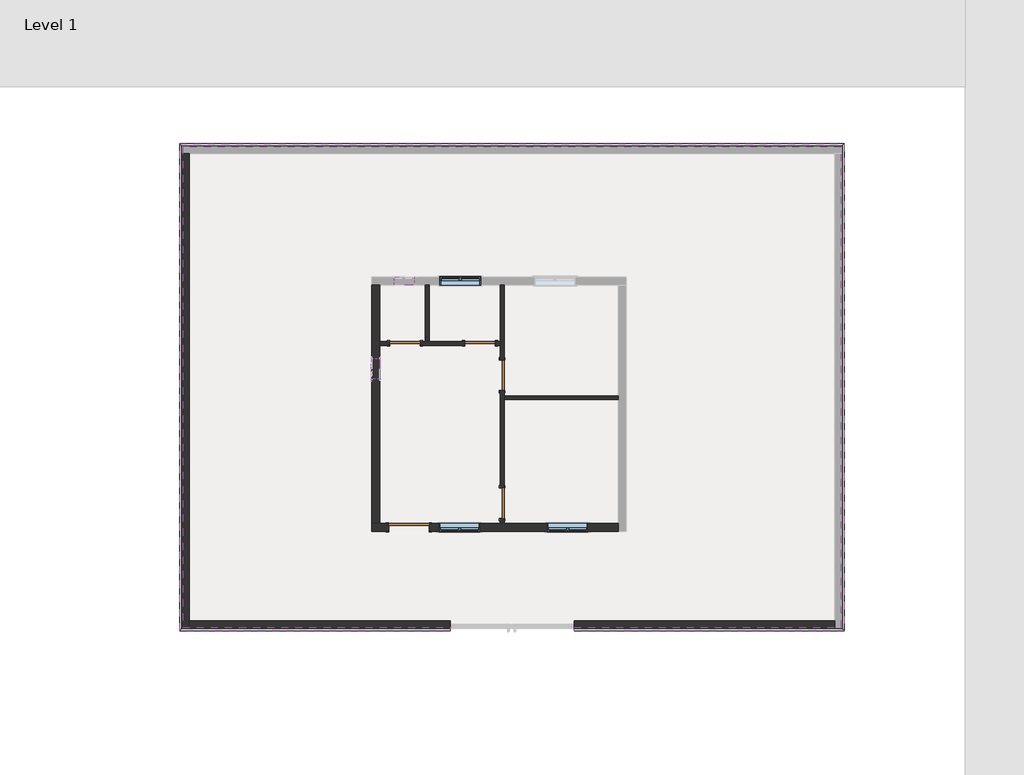
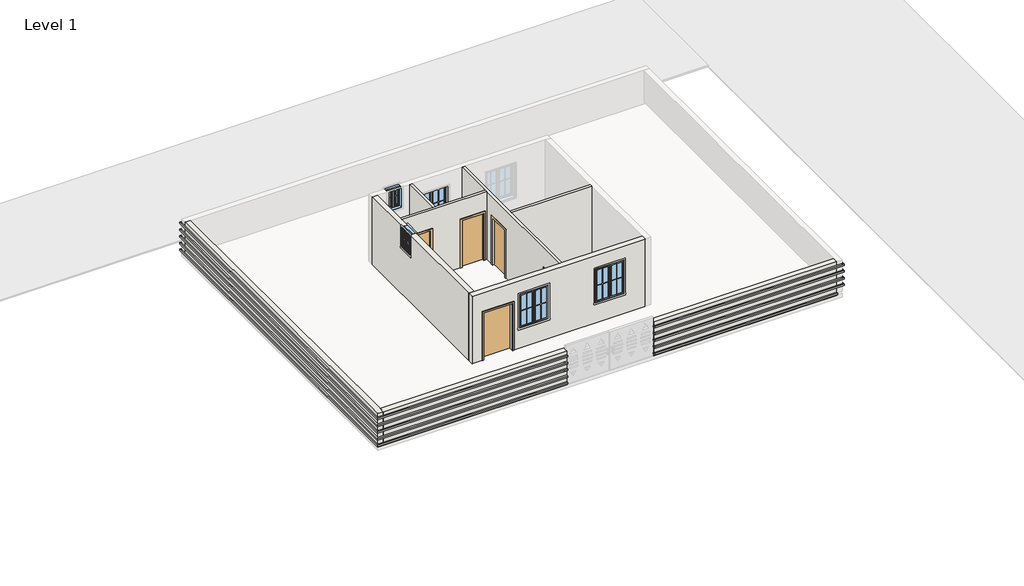
# One storey, part 1 of 2: 9 walls, 5 doors, 5 proxies, 5 windows.
"""IFC4 building model written with IfcOpenShell, lengths in millimetres."""

from ifc_helpers import new_model, si_unit, frame, origin, origin_with_axes, place, context, project, spatial, polyline, outline, extrude, faceted_brep, transform, mapped, element, save
from components import door_e5f9f3c4, door_f4c4cdf2, window_c417fced, window_8377141f

model = new_model("IFC4")

# Units and contexts
model_context = context("Model", 3, world=origin())
ifc_project = project(units=[si_unit("LENGTHUNIT", "METRE", prefix="MILLI")], contexts=[model_context])

# Site, building, storey
site = spatial("IfcSite", under=ifc_project)
building = spatial("IfcBuilding", under=site)
storey = spatial("IfcBuildingStorey", under=building, Name="Level 1", Elevation=0.0)

# Proxies
placement = place(None, origin())
element("IfcBuildingElementProxy", 1, Name="Reveal", ObjectType="Reveal", at=placement, inside=storey, context=model_context, shape_type="SweptSolid", body=[
    extrude(outline(polyline([(3367.5654616, 3455.855505), (3367.5654616, 3363.780505), (-4756.9239856, 3363.780505), (-4664.8489856, 3455.855505), (3367.5654616, 3455.855505)])), frame((0.0, 0.0, 76.2), z_axis=(0.0, 0.0, 1.0), x_axis=(1.0, 0.0, 0.0)), (0.0, 0.0, 1.0), 67.7333333),
    extrude(outline(polyline([(14893.1510144, 3455.855505), (14893.1510144, 3363.780505), (7082.6510144, 3363.780505), (7082.6510144, 3455.855505), (14893.1510144, 3455.855505)])), frame((0.0, 0.0, 76.2), z_axis=(0.0, 0.0, 1.0), x_axis=(1.0, 0.0, 0.0)), (0.0, 0.0, 1.0), 67.7333333),
    extrude(outline(polyline([(-4664.8489856, 17883.055505), (-4756.9239856, 17975.130505), (15121.7510144, 17975.130505), (15121.7510144, 17883.055505), (-4664.8489856, 17883.055505)])), frame((0.0, 0.0, 76.2), z_axis=(0.0, 0.0, 1.0), x_axis=(1.0, 0.0, 0.0)), (0.0, 0.0, 1.0), 67.7333333),
    extrude(outline(polyline([(-4664.8489856, 3455.855505), (-4756.9239856, 3363.780505), (-4756.9239856, 17975.130505), (-4664.8489856, 17883.055505), (-4664.8489856, 3455.855505)])), frame((0.0, 0.0, 76.2), z_axis=(0.0, 0.0, 1.0), x_axis=(1.0, 0.0, 0.0)), (0.0, 0.0, 1.0), 67.7333333),
])
element("IfcBuildingElementProxy", 2, Name="Reveal", ObjectType="Reveal", at=placement, inside=storey, context=model_context, shape_type="SweptSolid", body=[
    extrude(outline(polyline([(3367.5654616, 3455.855505), (3367.5654616, 3363.780505), (-4756.9239856, 3363.780505), (-4664.8489856, 3455.855505), (3367.5654616, 3455.855505)])), frame((0.0, 0.0, 381.0), z_axis=(0.0, 0.0, 1.0), x_axis=(1.0, 0.0, 0.0)), (0.0, 0.0, 1.0), 67.7333333),
    extrude(outline(polyline([(15096.3510144, 3455.855505), (15188.4260144, 3363.780505), (7082.6510144, 3363.780505), (7082.6510144, 3455.855505), (15096.3510144, 3455.855505)])), frame((0.0, 0.0, 381.0), z_axis=(0.0, 0.0, 1.0), x_axis=(1.0, 0.0, 0.0)), (0.0, 0.0, 1.0), 67.7333333),
    extrude(outline(polyline([(15096.3510144, 17883.055505), (15188.4260144, 17975.130505), (15188.4260144, 3363.780505), (15096.3510144, 3455.855505), (15096.3510144, 17883.055505)])), frame((0.0, 0.0, 381.0), z_axis=(0.0, 0.0, 1.0), x_axis=(1.0, 0.0, 0.0)), (0.0, 0.0, 1.0), 67.7333333),
    extrude(outline(polyline([(-4664.8489856, 17883.055505), (-4756.9239856, 17975.130505), (15188.4260144, 17975.130505), (15096.3510144, 17883.055505), (-4664.8489856, 17883.055505)])), frame((0.0, 0.0, 381.0), z_axis=(0.0, 0.0, 1.0), x_axis=(1.0, 0.0, 0.0)), (0.0, 0.0, 1.0), 67.7333333),
    extrude(outline(polyline([(-4664.8489856, 3455.855505), (-4756.9239856, 3363.780505), (-4756.9239856, 17975.130505), (-4664.8489856, 17883.055505), (-4664.8489856, 3455.855505)])), frame((0.0, 0.0, 381.0), z_axis=(0.0, 0.0, 1.0), x_axis=(1.0, 0.0, 0.0)), (0.0, 0.0, 1.0), 67.7333333),
])
element("IfcBuildingElementProxy", 3, Name="Reveal", ObjectType="Reveal", at=placement, inside=storey, context=model_context, shape_type="SweptSolid", body=[
    extrude(outline(polyline([(3367.5654616, 3455.855505), (3367.5654616, 3363.780505), (-4756.9239856, 3363.780505), (-4664.8489856, 3455.855505), (3367.5654616, 3455.855505)])), frame((0.0, 0.0, 685.8), z_axis=(0.0, 0.0, 1.0), x_axis=(1.0, 0.0, 0.0)), (0.0, 0.0, 1.0), 67.7333333),
    extrude(outline(polyline([(15096.3510144, 3455.855505), (15188.4260144, 3363.780505), (7082.6510144, 3363.780505), (7082.6510144, 3455.855505), (15096.3510144, 3455.855505)])), frame((0.0, 0.0, 685.8), z_axis=(0.0, 0.0, 1.0), x_axis=(1.0, 0.0, 0.0)), (0.0, 0.0, 1.0), 67.7333333),
    extrude(outline(polyline([(15096.3510144, 17883.055505), (15188.4260144, 17975.130505), (15188.4260144, 3363.780505), (15096.3510144, 3455.855505), (15096.3510144, 17883.055505)])), frame((0.0, 0.0, 685.8), z_axis=(0.0, 0.0, 1.0), x_axis=(1.0, 0.0, 0.0)), (0.0, 0.0, 1.0), 67.7333333),
    extrude(outline(polyline([(-4664.8489856, 17883.055505), (-4756.9239856, 17975.130505), (15188.4260144, 17975.130505), (15096.3510144, 17883.055505), (-4664.8489856, 17883.055505)])), frame((0.0, 0.0, 685.8), z_axis=(0.0, 0.0, 1.0), x_axis=(1.0, 0.0, 0.0)), (0.0, 0.0, 1.0), 67.7333333),
    extrude(outline(polyline([(-4664.8489856, 3455.855505), (-4756.9239856, 3363.780505), (-4756.9239856, 17975.130505), (-4664.8489856, 17883.055505), (-4664.8489856, 3455.855505)])), frame((0.0, 0.0, 685.8), z_axis=(0.0, 0.0, 1.0), x_axis=(1.0, 0.0, 0.0)), (0.0, 0.0, 1.0), 67.7333333),
])
element("IfcBuildingElementProxy", 4, Name="Reveal", ObjectType="Reveal", at=placement, inside=storey, context=model_context, shape_type="SweptSolid", body=[
    extrude(outline(polyline([(3367.5654616, 3455.855505), (3367.5654616, 3363.780505), (-4756.9239856, 3363.780505), (-4664.8489856, 3455.855505), (3367.5654616, 3455.855505)])), frame((0.0, 0.0, 990.6), z_axis=(0.0, 0.0, 1.0), x_axis=(1.0, 0.0, 0.0)), (0.0, 0.0, 1.0), 67.7333333),
    extrude(outline(polyline([(15096.3510144, 3455.855505), (15188.4260144, 3363.780505), (7082.6510144, 3363.780505), (7082.6510144, 3455.855505), (15096.3510144, 3455.855505)])), frame((0.0, 0.0, 990.6), z_axis=(0.0, 0.0, 1.0), x_axis=(1.0, 0.0, 0.0)), (0.0, 0.0, 1.0), 67.7333333),
    extrude(outline(polyline([(15096.3510144, 17883.055505), (15188.4260144, 17975.130505), (15188.4260144, 3363.780505), (15096.3510144, 3455.855505), (15096.3510144, 17883.055505)])), frame((0.0, 0.0, 990.6), z_axis=(0.0, 0.0, 1.0), x_axis=(1.0, 0.0, 0.0)), (0.0, 0.0, 1.0), 67.7333333),
    extrude(outline(polyline([(-4664.8489856, 17883.055505), (-4756.9239856, 17975.130505), (15188.4260144, 17975.130505), (15096.3510144, 17883.055505), (-4664.8489856, 17883.055505)])), frame((0.0, 0.0, 990.6), z_axis=(0.0, 0.0, 1.0), x_axis=(1.0, 0.0, 0.0)), (0.0, 0.0, 1.0), 67.7333333),
    extrude(outline(polyline([(-4664.8489856, 3455.855505), (-4756.9239856, 3363.780505), (-4756.9239856, 17975.130505), (-4664.8489856, 17883.055505), (-4664.8489856, 3455.855505)])), frame((0.0, 0.0, 990.6), z_axis=(0.0, 0.0, 1.0), x_axis=(1.0, 0.0, 0.0)), (0.0, 0.0, 1.0), 67.7333333),
])
element("IfcBuildingElementProxy", 5, Name="Reveal", ObjectType="Reveal", at=placement, inside=storey, context=model_context, shape_type="SweptSolid", body=[
    extrude(outline(polyline([(3367.5654616, 3455.855505), (3367.5654616, 3363.780505), (-4756.9239856, 3363.780505), (-4664.8489856, 3455.855505), (3367.5654616, 3455.855505)])), frame((0.0, 0.0, 1295.4), z_axis=(0.0, 0.0, 1.0), x_axis=(1.0, 0.0, 0.0)), (0.0, 0.0, 1.0), 67.7333333),
    extrude(outline(polyline([(15096.3510144, 3455.855505), (15188.4260144, 3363.780505), (7082.6510144, 3363.780505), (7082.6510144, 3455.855505), (15096.3510144, 3455.855505)])), frame((0.0, 0.0, 1295.4), z_axis=(0.0, 0.0, 1.0), x_axis=(1.0, 0.0, 0.0)), (0.0, 0.0, 1.0), 67.7333333),
    extrude(outline(polyline([(15096.3510144, 17883.055505), (15188.4260144, 17975.130505), (15188.4260144, 3363.780505), (15096.3510144, 3455.855505), (15096.3510144, 17883.055505)])), frame((0.0, 0.0, 1295.4), z_axis=(0.0, 0.0, 1.0), x_axis=(1.0, 0.0, 0.0)), (0.0, 0.0, 1.0), 67.7333333),
    extrude(outline(polyline([(-4664.8489856, 17883.055505), (-4756.9239856, 17975.130505), (15188.4260144, 17975.130505), (15096.3510144, 17883.055505), (-4664.8489856, 17883.055505)])), frame((0.0, 0.0, 1295.4), z_axis=(0.0, 0.0, 1.0), x_axis=(1.0, 0.0, 0.0)), (0.0, 0.0, 1.0), 67.7333333),
    extrude(outline(polyline([(-4664.8489856, 3455.855505), (-4756.9239856, 3363.780505), (-4756.9239856, 17975.130505), (-4664.8489856, 17883.055505), (-4664.8489856, 3455.855505)])), frame((0.0, 0.0, 1295.4), z_axis=(0.0, 0.0, 1.0), x_axis=(1.0, 0.0, 0.0)), (0.0, 0.0, 1.0), 67.7333333),
])

# Doors
door_shape = door_e5f9f3c4(model_context)
element("IfcDoor", 6, ObjectType="Single-Flush : 36\" x 84\"", at=placement, inside=storey, context=model_context, shape_type="MappedRepresentation", body=[
    mapped(door_shape, transform((2006.6, 11982.45, 0.0), x_axis=(1.0, 0.0, 0.0), y_axis=(0.0, 1.0, 0.0), z_axis=(0.0, 0.0, 1.0))),
])
element("IfcDoor", 7, ObjectType="Single-Flush : 36\" x 84\"", at=placement, inside=storey, context=model_context, shape_type="MappedRepresentation", body=[
    mapped(door_shape, transform((4254.5, 11982.45, 0.0), x_axis=(1.0, 0.0, 0.0), y_axis=(0.0, 1.0, 0.0), z_axis=(0.0, 0.0, 1.0))),
])
element("IfcDoor", 8, ObjectType="Single-Flush : 36\" x 84\"", at=placement, inside=storey, context=model_context, shape_type="MappedRepresentation", body=[
    mapped(door_shape, transform((4921.25, 11023.6, 0.0), x_axis=(0.0, -1.0, 0.0), y_axis=(1.0, 0.0, 0.0), z_axis=(0.0, 0.0, 1.0))),
])
element("IfcDoor", 9, ObjectType="Single-Flush : 36\" x 84\"", at=placement, inside=storey, context=model_context, shape_type="MappedRepresentation", body=[
    mapped(door_shape, transform((4921.25, 7188.2, 0.0), x_axis=(0.0, -1.0, 0.0), y_axis=(1.0, 0.0, 0.0), z_axis=(0.0, 0.0, 1.0))),
])
door_2_shape = door_f4c4cdf2(model_context)
element("IfcDoor", 10, ObjectType="Single-Flush : 48\" x 84\"", at=placement, inside=storey, context=model_context, shape_type="MappedRepresentation", body=[
    mapped(door_2_shape, transform((2120.9, 6464.3, 0.0), x_axis=(-1.0, 0.0, 0.0), y_axis=(0.0, -1.0, 0.0), z_axis=(0.0, 0.0, 1.0))),
])

# Walls
element("IfcWall", 11, ObjectType="Generic - 5\"", at=placement, inside=storey, context=model_context, shape_type="SweptSolid", body=[
    extrude(outline(polyline([(2616.2, 12039.6), (2616.2, 13741.4), (2730.5, 13741.4), (2730.5, 12039.6), (2616.2, 12039.6)])), origin_with_axes(), (0.0, 0.0, 1.0), 3048.0),
])
element("IfcWall", 12, ObjectType="Generic - 5\"", at=placement, inside=storey, context=model_context, shape_type="Brep", body=[
    faceted_brep([(4711.7, 11925.3, 2133.6), (4711.7, 11925.3, 0.0), (4864.1, 11925.3, 0.0), (4864.1, 11925.3, 3048.0), (1244.6, 11925.3, 3048.0), (1244.6, 11925.3, 0.0), (1549.4, 11925.3, 0.0), (1549.4, 11925.3, 2133.6), (2463.8, 11925.3, 2133.6), (2463.8, 11925.3, 0.0), (3797.3, 11925.3, 0.0), (3797.3, 11925.3, 2133.6), (4864.1, 12039.6, 0.0), (4711.7, 12039.6, 0.0), (4711.7, 12039.6, 2133.6), (3797.3, 12039.6, 2133.6), (3797.3, 12039.6, 0.0), (2730.5, 12039.6, 0.0), (2616.2, 12039.6, 0.0), (2463.8, 12039.6, 0.0), (2463.8, 12039.6, 2133.6), (1549.4, 12039.6, 2133.6), (1549.4, 12039.6, 0.0), (1244.6, 12039.6, 0.0), (1244.6, 12039.6, 3048.0), (2616.2, 12039.6, 3048.0), (2730.5, 12039.6, 3048.0), (4864.1, 12039.6, 3048.0)], [[[0, 1, 2, 3, 4, 5, 6, 7, 8, 9, 10, 11]], [[12, 13, 14, 15, 16, 17, 18, 19, 20, 21, 22, 23, 24, 25, 26, 27]], [[6, 5, 23, 22]], [[10, 9, 19, 18, 17, 16]], [[2, 1, 13, 12]], [[4, 3, 27, 26, 25, 24]], [[5, 4, 24, 23]], [[3, 2, 12, 27]], [[20, 19, 9, 8]], [[21, 20, 8, 7]], [[22, 21, 7, 6]], [[14, 13, 1, 0]], [[15, 14, 0, 11]], [[16, 15, 11, 10]]]),
])
element("IfcWall", 13, ObjectType="Generic - 5\"", at=placement, inside=storey, context=model_context, shape_type="Brep", body=[
    faceted_brep([(4864.1, 6731.0, 2133.6), (4864.1, 6731.0, 0.0), (4864.1, 6578.6, 0.0), (4864.1, 6578.6, 3048.0), (4864.1, 11925.3, 3048.0), (4864.1, 12039.6, 3048.0), (4864.1, 13741.4, 3048.0), (4864.1, 13741.4, 0.0), (4864.1, 12039.6, 0.0), (4864.1, 11925.3, 0.0), (4864.1, 11480.8, 0.0), (4864.1, 11480.8, 2133.6), (4864.1, 10566.4, 2133.6), (4864.1, 10566.4, 0.0), (4864.1, 7645.4, 0.0), (4864.1, 7645.4, 2133.6), (4978.4, 6578.6, 0.0), (4978.4, 6731.0, 0.0), (4978.4, 6731.0, 2133.6), (4978.4, 7645.4, 2133.6), (4978.4, 7645.4, 0.0), (4978.4, 10299.7, 0.0), (4978.4, 10414.0, 0.0), (4978.4, 10566.4, 0.0), (4978.4, 10566.4, 2133.6), (4978.4, 11480.8, 2133.6), (4978.4, 11480.8, 0.0), (4978.4, 13741.4, 0.0), (4978.4, 13741.4, 3048.0), (4978.4, 10414.0, 3048.0), (4978.4, 10299.7, 3048.0), (4978.4, 6578.6, 3048.0)], [[[0, 1, 2, 3, 4, 5, 6, 7, 8, 9, 10, 11, 12, 13, 14, 15]], [[16, 17, 18, 19, 20, 21, 22, 23, 24, 25, 26, 27, 28, 29, 30, 31]], [[10, 9, 8, 7, 27, 26]], [[14, 13, 23, 22, 21, 20]], [[2, 1, 17, 16]], [[6, 5, 4, 3, 31, 30, 29, 28]], [[7, 6, 28, 27]], [[3, 2, 16, 31]], [[24, 23, 13, 12]], [[25, 24, 12, 11]], [[26, 25, 11, 10]], [[18, 17, 1, 0]], [[19, 18, 0, 15]], [[20, 19, 15, 14]]]),
])
element("IfcWall", 14, ObjectType="Generic - 5\"", at=placement, inside=storey, context=model_context, shape_type="SweptSolid", body=[
    extrude(outline(polyline([(8407.4, 10299.7), (4978.4, 10299.7), (4978.4, 10414.0), (8407.4, 10414.0), (8407.4, 10299.7)])), origin_with_axes(), (0.0, 0.0, 1.0), 3048.0),
])
element("IfcWall", 15, ObjectType="Generic - 8\"", at=placement, inside=storey, context=model_context, shape_type="Brep", body=[
    faceted_brep([(1511.3, 6578.6, 2133.6), (1511.3, 6578.6, 0.0), (1244.6, 6578.6, 0.0), (1016.0, 6578.6, 0.0), (1016.0, 6578.6, 3048.0), (1244.6, 6578.6, 3048.0), (4864.1, 6578.6, 3048.0), (4978.4, 6578.6, 3048.0), (8407.4, 6578.6, 3048.0), (8407.4, 6578.6, 0.0), (4978.4, 6578.6, 0.0), (4864.1, 6578.6, 0.0), (2730.5, 6578.6, 0.0), (2730.5, 6578.6, 2133.6), (6273.8, 6578.6, 2438.4), (6273.8, 6578.6, 914.4), (7493.0, 6578.6, 914.4), (7493.0, 6578.6, 2438.4), (3035.3, 6578.6, 2438.4), (3035.3, 6578.6, 914.4), (4254.5, 6578.6, 914.4), (4254.5, 6578.6, 2438.4), (1016.0, 6350.0, 0.0), (1511.3, 6350.0, 0.0), (1511.3, 6350.0, 2133.6), (2730.5, 6350.0, 2133.6), (2730.5, 6350.0, 0.0), (8407.4, 6350.0, 0.0), (8407.4, 6350.0, 3048.0), (1016.0, 6350.0, 3048.0), (6273.8, 6350.0, 2438.4), (7493.0, 6350.0, 2438.4), (7493.0, 6350.0, 914.4), (6273.8, 6350.0, 914.4), (3035.3, 6350.0, 2438.4), (4254.5, 6350.0, 2438.4), (4254.5, 6350.0, 914.4), (3035.3, 6350.0, 914.4)], [[[0, 1, 2, 3, 4, 5, 6, 7, 8, 9, 10, 11, 12, 13], [14, 15, 16, 17], [18, 19, 20, 21]], [[22, 23, 24, 25, 26, 27, 28, 29], [30, 31, 32, 33], [34, 35, 36, 37]], [[3, 2, 1, 23, 22]], [[12, 11, 10, 9, 27, 26]], [[9, 8, 28, 27]], [[4, 3, 22, 29]], [[24, 23, 1, 0]], [[25, 24, 0, 13]], [[26, 25, 13, 12]], [[15, 14, 30, 33]], [[16, 15, 33, 32]], [[17, 16, 32, 31]], [[14, 17, 31, 30]], [[19, 18, 34, 37]], [[20, 19, 37, 36]], [[21, 20, 36, 35]], [[18, 21, 35, 34]], [[8, 7, 6, 5, 4, 29, 28]]]),
])
element("IfcWall", 16, ObjectType="Generic - 8\"", at=placement, inside=storey, context=model_context, shape_type="Brep", body=[
    faceted_brep([(1244.6, 6578.6, 0.0), (1244.6, 11925.3, 0.0), (1244.6, 12039.6, 0.0), (1244.6, 13741.4, 0.0), (1244.6, 13741.4, 3048.0), (1244.6, 12039.6, 3048.0), (1244.6, 11925.3, 3048.0), (1244.6, 11525.25, 3048.0), (1244.6, 11525.25, 2133.6), (1244.6, 10915.65, 2133.6), (1244.6, 10915.65, 3048.0), (1244.6, 6578.6, 3048.0), (1016.0, 13741.4, 0.0), (1016.0, 6578.6, 0.0), (1016.0, 6578.6, 3048.0), (1016.0, 10915.65, 3048.0), (1016.0, 10915.65, 2133.6), (1016.0, 11525.25, 2133.6), (1016.0, 11525.25, 3048.0), (1016.0, 13741.4, 3048.0)], [[[0, 1, 2, 3, 4, 5, 6, 7, 8, 9, 10, 11]], [[12, 13, 14, 15, 16, 17, 18, 19]], [[3, 2, 1, 0, 13, 12]], [[4, 3, 12, 19]], [[0, 11, 14, 13]], [[14, 11, 10, 15]], [[4, 19, 18, 7, 6, 5]], [[17, 8, 7, 18]], [[8, 17, 16, 9]], [[9, 16, 15, 10]]]),
])
element("IfcWall", 17, ObjectType="Generic - 8\"", at=placement, inside=storey, context=model_context, shape_type="SweptSolid", body=[
    extrude(outline(polyline([(3659.055505, 1524.0), (3659.055505, 0.0), (3430.455505, 0.0), (3430.455505, 76.2), (3455.855505, 76.2), (3455.855505, 143.9333333), (3430.455505, 143.9333333), (3430.455505, 381.0), (3455.855505, 381.0), (3455.855505, 448.7333333), (3430.455505, 448.7333333), (3430.455505, 685.8), (3455.855505, 685.8), (3455.855505, 753.5333333), (3430.455505, 753.5333333), (3430.455505, 990.6), (3455.855505, 990.6), (3455.855505, 1058.3333333), (3430.455505, 1058.3333333), (3430.455505, 1295.4), (3455.855505, 1295.4), (3455.855505, 1363.1333333), (3430.455505, 1363.1333333), (3430.455505, 1524.0), (3659.055505, 1524.0)])), frame((7082.6510144, 0.0, 0.0), z_axis=(1.0, 0.0, 0.0), x_axis=(0.0, 1.0, 0.0)), (0.0, 0.0, 1.0), 7810.5),
])
element("IfcWall", 18, ObjectType="Generic - 8\"", at=placement, inside=storey, context=model_context, shape_type="Brep", body=[
    faceted_brep([(-4461.6489856, 3430.455505, 0.0), (-4461.6489856, 3659.055505, 0.0), (-4461.6489856, 17679.855505, 0.0), (-4461.6489856, 17679.855505, 1524.0), (-4461.6489856, 3659.055505, 1524.0), (-4461.6489856, 3430.455505, 1524.0), (-4461.6489856, 3430.455505, 1363.1333333), (-4461.6489856, 3455.855505, 1363.1333333), (-4461.6489856, 3455.855505, 1295.4), (-4461.6489856, 3430.455505, 1295.4), (-4461.6489856, 3430.455505, 1058.3333333), (-4461.6489856, 3455.855505, 1058.3333333), (-4461.6489856, 3455.855505, 990.6), (-4461.6489856, 3430.455505, 990.6), (-4461.6489856, 3430.455505, 753.5333333), (-4461.6489856, 3455.855505, 753.5333333), (-4461.6489856, 3455.855505, 685.8), (-4461.6489856, 3430.455505, 685.8), (-4461.6489856, 3430.455505, 448.7333333), (-4461.6489856, 3455.855505, 448.7333333), (-4461.6489856, 3455.855505, 381.0), (-4461.6489856, 3430.455505, 381.0), (-4461.6489856, 3430.455505, 143.9333333), (-4461.6489856, 3455.855505, 143.9333333), (-4461.6489856, 3455.855505, 76.2), (-4461.6489856, 3430.455505, 76.2), (-4690.2489856, 17679.855505, 0.0), (-4690.2489856, 3430.455505, 0.0), (-4690.2489856, 3430.455505, 76.2), (-4690.2489856, 17679.855505, 76.2), (-4690.2489856, 3430.455505, 1524.0), (-4690.2489856, 17679.855505, 1524.0), (-4690.2489856, 17679.855505, 1363.1333333), (-4690.2489856, 3430.455505, 1363.1333333), (-4690.2489856, 17679.855505, 143.9333333), (-4690.2489856, 3430.455505, 143.9333333), (-4690.2489856, 3430.455505, 381.0), (-4690.2489856, 17679.855505, 381.0), (-4690.2489856, 17679.855505, 448.7333333), (-4690.2489856, 3430.455505, 448.7333333), (-4690.2489856, 3430.455505, 685.8), (-4690.2489856, 17679.855505, 685.8), (-4690.2489856, 17679.855505, 753.5333333), (-4690.2489856, 3430.455505, 753.5333333), (-4690.2489856, 3430.455505, 990.6), (-4690.2489856, 17679.855505, 990.6), (-4690.2489856, 17679.855505, 1058.3333333), (-4690.2489856, 3430.455505, 1058.3333333), (-4690.2489856, 3430.455505, 1295.4), (-4690.2489856, 17679.855505, 1295.4), (-4664.8489856, 17679.855505, 76.2), (-4664.8489856, 17679.855505, 143.9333333), (-4664.8489856, 17679.855505, 381.0), (-4664.8489856, 17679.855505, 448.7333333), (-4664.8489856, 17679.855505, 685.8), (-4664.8489856, 17679.855505, 753.5333333), (-4664.8489856, 17679.855505, 990.6), (-4664.8489856, 17679.855505, 1058.3333333), (-4664.8489856, 17679.855505, 1295.4), (-4664.8489856, 17679.855505, 1363.1333333), (-4664.8489856, 3455.855505, 143.9333333), (-4664.8489856, 3455.855505, 76.2), (-4664.8489856, 3455.855505, 448.7333333), (-4664.8489856, 3455.855505, 381.0), (-4664.8489856, 3455.855505, 753.5333333), (-4664.8489856, 3455.855505, 685.8), (-4664.8489856, 3455.855505, 1058.3333333), (-4664.8489856, 3455.855505, 990.6), (-4664.8489856, 3455.855505, 1363.1333333), (-4664.8489856, 3455.855505, 1295.4)], [[[0, 1, 2, 3, 4, 5, 6, 7, 8, 9, 10, 11, 12, 13, 14, 15, 16, 17, 18, 19, 20, 21, 22, 23, 24, 25]], [[26, 27, 28, 29]], [[30, 31, 32, 33]], [[34, 35, 36, 37]], [[38, 39, 40, 41]], [[42, 43, 44, 45]], [[46, 47, 48, 49]], [[2, 1, 0, 27, 26]], [[5, 4, 3, 31, 30]], [[3, 2, 26, 29, 50, 51, 34, 37, 52, 53, 38, 41, 54, 55, 42, 45, 56, 57, 46, 49, 58, 59, 32, 31]], [[5, 30, 33, 6]], [[27, 0, 25, 28]], [[35, 22, 21, 36]], [[39, 18, 17, 40]], [[43, 14, 13, 44]], [[47, 10, 9, 48]], [[51, 60, 23, 22, 35, 34]], [[24, 61, 50, 29, 28, 25]], [[60, 61, 24, 23]], [[61, 60, 51, 50]], [[53, 62, 19, 18, 39, 38]], [[20, 63, 52, 37, 36, 21]], [[62, 63, 20, 19]], [[63, 62, 53, 52]], [[55, 64, 15, 14, 43, 42]], [[16, 65, 54, 41, 40, 17]], [[64, 65, 16, 15]], [[65, 64, 55, 54]], [[57, 66, 11, 10, 47, 46]], [[12, 67, 56, 45, 44, 13]], [[66, 67, 12, 11]], [[67, 66, 57, 56]], [[59, 68, 7, 6, 33, 32]], [[8, 69, 58, 49, 48, 9]], [[68, 69, 8, 7]], [[69, 68, 59, 58]]]),
])
element("IfcWall", 19, ObjectType="Generic - 8\"", at=placement, inside=storey, context=model_context, shape_type="SweptSolid", body=[
    extrude(outline(polyline([(3659.055505, 1524.0), (3659.055505, 0.0), (3430.455505, 0.0), (3430.455505, 76.2), (3455.855505, 76.2), (3455.855505, 143.9333333), (3430.455505, 143.9333333), (3430.455505, 381.0), (3455.855505, 381.0), (3455.855505, 448.7333333), (3430.455505, 448.7333333), (3430.455505, 685.8), (3455.855505, 685.8), (3455.855505, 753.5333333), (3430.455505, 753.5333333), (3430.455505, 990.6), (3455.855505, 990.6), (3455.855505, 1058.3333333), (3430.455505, 1058.3333333), (3430.455505, 1295.4), (3455.855505, 1295.4), (3455.855505, 1363.1333333), (3430.455505, 1363.1333333), (3430.455505, 1524.0), (3659.055505, 1524.0)])), frame((-4461.6489856, 0.0, 0.0), z_axis=(1.0, 0.0, 0.0), x_axis=(0.0, 1.0, 0.0)), (0.0, 0.0, 1.0), 7829.2144471),
])

# Windows
window_shape = window_c417fced(model_context)
element("IfcWindow", 20, ObjectType="Window-Casement-Double : 24\" x 36\"", at=placement, inside=storey, context=model_context, shape_type="MappedRepresentation", body=[
    mapped(window_shape, transform((1130.3, 11220.45, 1219.2), x_axis=(0.0, 1.0, 0.0), y_axis=(-1.0, 0.0, 0.0), z_axis=(0.0, 0.0, 1.0))),
])
element("IfcWindow", 21, ObjectType="Window-Casement-Double : 24\" x 36\"", at=placement, inside=storey, context=model_context, shape_type="MappedRepresentation", body=[
    mapped(window_shape, transform((1981.2, 13855.7, 1219.2), x_axis=(1.0, 0.0, 0.0), y_axis=(0.0, 1.0, 0.0), z_axis=(0.0, 0.0, 1.0))),
])
window_2_shape = window_8377141f(model_context)
element("IfcWindow", 22, ObjectType="Window-Casement-Double : 48\" x 60\"", at=placement, inside=storey, context=model_context, shape_type="MappedRepresentation", body=[
    mapped(window_2_shape, transform((6883.4, 6464.3, 0.0), x_axis=(-1.0, 0.0, 0.0), y_axis=(0.0, -1.0, 0.0), z_axis=(0.0, 0.0, 1.0))),
])
element("IfcWindow", 23, ObjectType="Window-Casement-Double : 48\" x 60\"", at=placement, inside=storey, context=model_context, shape_type="MappedRepresentation", body=[
    mapped(window_2_shape, transform((3644.9, 6464.3, 0.0), x_axis=(-1.0, 0.0, 0.0), y_axis=(0.0, -1.0, 0.0), z_axis=(0.0, 0.0, 1.0))),
])
element("IfcWindow", 24, ObjectType="Window-Casement-Double : 48\" x 60\"", at=placement, inside=storey, context=model_context, shape_type="MappedRepresentation", body=[
    mapped(window_2_shape, transform((3663.95, 13855.7, 0.0), x_axis=(1.0, 0.0, 0.0), y_axis=(0.0, 1.0, 0.0), z_axis=(0.0, 0.0, 1.0))),
])

save(model, "model.ifc")

# Revit data of these elements
# Type "Single-Flush : 36\" x 84\""
#   Type Mark = "1"
#   Construction Type Id = "MDOOR"
#   Assembly Code = "C1020"
#   Analytic Construction = "Metal"
#   Thickness = 0' - 2"
#   Heat Transfer Coefficient (U) = 0.651978 BTU/(h·ft²·°F)
#   Height = 7' - 0"
#   Trim Projection Ext = 0' - 1"
#   Trim Projection Int = 0' - 1"
#   Trim Width = 0' - 3"
#   Width = 3' - 0"
#   Define Thermal Properties by = 1
#   Define Thermal Properties by = 1
#   Door Material = Door - Panel
#   Frame Material = Door - Frame
#   Visual Light Transmittance = 0
#   Solar Heat Gain Coefficient = 0
#   Function = (empty or 0)
#   Wall Closure = (empty or 0)
# Type "Single-Flush : 48\" x 84\""
#   Type Mark = "5"
#   Construction Type Id = "MDOOR"
#   Assembly Code = "C1020"
#   Analytic Construction = "Metal"
#   Thickness = 0' - 2"
#   Heat Transfer Coefficient (U) = 0.651978 BTU/(h·ft²·°F)
#   Height = 7' - 0"
#   Trim Projection Ext = 0' - 1"
#   Trim Projection Int = 0' - 1"
#   Trim Width = 0' - 3"
#   Width = 4' - 0"
#   Define Thermal Properties by = 1
#   Define Thermal Properties by = 1
#   Door Material = Door - Panel
#   Frame Material = Door - Frame
#   Visual Light Transmittance = 0
#   Solar Heat Gain Coefficient = 0
#   Function = (empty or 0)
#   Wall Closure = (empty or 0)
# Type "Generic - 5\""
#   Assembly Code = "B2010"
#   Layers, outside or top first: 0' - 4 1/2" no material (function 1)
# Type "Generic - 8\""
#   Assembly Code = "B2010"
#   Layers, outside or top first: 0' - 9" "Parking Stripe" (function 1)
# Type "Window-Casement-Double : 24\" x 36\""
#   Type Mark = "14"
#   Fire Rating = "0.5h"
#   Assembly Code = "B2020100"
#   Analytic Construction = "Double glazing - domestic"
#   Frame Extension [instance default] = 0' - 0 1/4"
#   Window Inset [instance default] = 0' - 0"
#   Wall Thickness [instance default] = 0' - 6"
#   Interior Wall Closure [instance default] = 0' - 2 1/4"
#   Half Width = 1' - 0"
#   Visual Light Transmittance = 0.81
#   Thermal Resistance (R) = 1.8146 (h·ft²·°F)/BTU
#   Solar Heat Gain Coefficient = 0.76
#   Rough Width = 2' - 0 1/2"
#   Rough Height = 3' - 0 1/2"
#   Height = 3' - 0"
#   Heat Transfer Coefficient (U) = 0.5511 BTU/(h·ft²·°F)
#   Exterior Wall Closure [instance default] = 0' - 1 1/4"
#   Extension Jamb [instance default] = 0' - 2 1/4"
#   Default Sill Height = 3' - 0"
#   Width = 2' - 0"
#   Define Thermal Properties by = 0
#   Muntin Visibility = yes
#   Interior Trim Visibility [instance default] = yes
#   Exterior Trim Visibility [instance default] = yes
#   Extension Jamb Visibility [instance default] = yes
#   Interior Trim Material = Wood - Stained
#   Muntin Pattern = Muntin Pattern_2x2 : Muntin Pattern_2x2
#   Interior Trim = Trim-Window-Interior-Flat : Picture Frame
#   Interior Frame Material = Wood - Stained
#   Glass Panel Material = Glass
#   Exterior Trim Material = Clad - White
#   Exterior Trim = Trim-Window-Exterior-Flat : with Sill
#   Exterior Frame Material = Clad - White
#   Wall Closure = (empty or 0)
# Type "Window-Casement-Double : 48\" x 60\""
#   Type Mark = "17"
#   Fire Rating = "0.5h"
#   Assembly Code = "B2020100"
#   Analytic Construction = "Double glazing - domestic"
#   Frame Extension [instance default] = 0' - 0 1/4"
#   Window Inset [instance default] = 0' - 0"
#   Wall Thickness [instance default] = 0' - 6"
#   Interior Wall Closure [instance default] = 0' - 2 1/4"
#   Half Width = 2' - 0"
#   Visual Light Transmittance = 0.81
#   Thermal Resistance (R) = 1.8146 (h·ft²·°F)/BTU
#   Solar Heat Gain Coefficient = 0.76
#   Rough Width = 4' - 0 1/2"
#   Rough Height = 5' - 0 1/2"
#   Height = 5' - 0"
#   Heat Transfer Coefficient (U) = 0.5511 BTU/(h·ft²·°F)
#   Exterior Wall Closure [instance default] = 0' - 1 1/4"
#   Extension Jamb [instance default] = 0' - 2 1/4"
#   Default Sill Height = 3' - 0"
#   Width = 4' - 0"
#   Define Thermal Properties by = 0
#   Muntin Visibility = yes
#   Interior Trim Visibility [instance default] = yes
#   Exterior Trim Visibility [instance default] = yes
#   Extension Jamb Visibility [instance default] = yes
#   Interior Trim Material = Wood - Stained
#   Muntin Pattern = Muntin Pattern_2x2 : Muntin Pattern_2x2
#   Interior Trim = Trim-Window-Interior-Flat : Picture Frame
#   Interior Frame Material = Wood - Stained
#   Glass Panel Material = Glass
#   Exterior Trim Material = Clad - White
#   Exterior Trim = Trim-Window-Exterior-Flat : with Sill
#   Exterior Frame Material = Clad - White
#   Wall Closure = (empty or 0)
# Elements 6, 7, 8, 9 (IfcDoor, "Single-Flush : 36\" x 84\"")
#   Phase Created = New Construction
#   Materials on its faces: "Door - Frame", "Door - Panel"
# Element 10 (IfcDoor, "Single-Flush : 48\" x 84\"")
#   Phase Created = New Construction
#   Materials on its faces: "Door - Frame", "Door - Panel"
# Elements 11, 12, 13, 14 (IfcWall, "Generic - 5\"")
#   Top Offset = 0' - 0"
#   Base Offset = 0' - 0"
#   wall height = 10' - 0"
#   Phase Created = New Construction
#   Base Constraint = Level 1
#   Top Constraint = Level 2
#   Materials on its faces: "Default Wall"
# Elements 15, 16 (IfcWall, "Generic - 8\"")
#   Top Offset = 0' - 0"
#   Base Offset = 0' - 0"
#   Unconnected Height = 10' - 0"
#   wall height = 10' - 0"
#   Phase Created = New Construction
#   Base Constraint = Level 1
#   Materials on its faces: "Parking Stripe", "Wood Planks"
# Elements 17, 18, 19 (IfcWall, "Generic - 8\"")
#   Top Offset = 0' - 0"
#   Base Offset = 0' - 0"
#   Unconnected Height = 5' - 0"
#   wall height = 5' - 0"
#   Phase Created = New Construction
#   Base Constraint = Level 1
#   Materials on its faces: "Parking Stripe", "Plywood, Sheathing", "Textile - Linen, Smooth"
# Element 20 (IfcWindow, "Window-Casement-Double : 24\" x 36\"")
#   Mark = "5"
#   Window Inset = 0' - 0"
#   Interior Wall Closure = 0' - 2 1/4"
#   Frame Extension = 0' - 0 1/4"
#   Exterior Wall Closure = 0' - 1 1/4"
#   Interior Trim Visibility = yes
#   Exterior Trim Visibility = yes
#   Phase Created = New Construction
#   Materials on its faces: "Wood - Stained", "Glass", "Clad - White"
# Element 21 (IfcWindow, "Window-Casement-Double : 24\" x 36\"")
#   Mark = "6"
#   Window Inset = 0' - 0"
#   Interior Wall Closure = 0' - 2 1/4"
#   Frame Extension = 0' - 0 1/4"
#   Exterior Wall Closure = 0' - 1 1/4"
#   Interior Trim Visibility = yes
#   Exterior Trim Visibility = yes
#   Phase Created = New Construction
#   Materials on its faces: "Wood - Stained", "Glass", "Clad - White"
# Element 22 (IfcWindow, "Window-Casement-Double : 48\" x 60\"")
#   Mark = "2"
#   Window Inset = 0' - 0"
#   Interior Wall Closure = 0' - 2 1/4"
#   Frame Extension = 0' - 0 1/4"
#   Exterior Wall Closure = 0' - 1 1/4"
#   Interior Trim Visibility = yes
#   Exterior Trim Visibility = yes
#   Phase Created = New Construction
#   Materials on its faces: "Wood - Stained", "Glass", "Clad - White"
# Element 23 (IfcWindow, "Window-Casement-Double : 48\" x 60\"")
#   Mark = "3"
#   Window Inset = 0' - 0"
#   Interior Wall Closure = 0' - 2 1/4"
#   Frame Extension = 0' - 0 1/4"
#   Exterior Wall Closure = 0' - 1 1/4"
#   Interior Trim Visibility = yes
#   Exterior Trim Visibility = yes
#   Phase Created = New Construction
#   Materials on its faces: "Wood - Stained", "Glass", "Clad - White"
# Element 24 (IfcWindow, "Window-Casement-Double : 48\" x 60\"")
#   Mark = "4"
#   Window Inset = 0' - 0"
#   Interior Wall Closure = 0' - 2 1/4"
#   Frame Extension = 0' - 0 1/4"
#   Exterior Wall Closure = 0' - 1 1/4"
#   Interior Trim Visibility = yes
#   Exterior Trim Visibility = yes
#   Phase Created = New Construction
#   Materials on its faces: "Wood - Stained", "Glass", "Clad - White"
# Materials
#   "Door - Panel": class "Wood", colour RGB 210 159 95, transparency 0, Cost = 0
#   "Door - Frame": colour RGB 118 70 51, transparency 0, Cost = 0
#   "Parking Stripe": class "Paint", colour RGB 250 250 91, transparency 0, Cost = 0
#   "Wood - Stained": class "Wood", colour RGB 224 178 126, transparency 0, Cost = 0
#   "Glass": class "Glass", colour RGB 0 128 192, transparency 0.75, Description = "Soda Lime Glass", Cost = 0
#   "Clad - White": class "Wood", colour RGB 242 242 238, transparency 0, Cost = 0
#   "Default Wall": colour RGB 128 128 128, transparency 0, Cost = 0
#   "Wood Planks": class "Wood", colour RGB 193 160 115, transparency 0, Description = "Physical material.", Cost = 0
#   "Plywood, Sheathing": class "Wood", colour RGB 212 179 113, transparency 0, Description = "Plywood, sheathing grade", Cost = 0
#   "Textile - Linen, Smooth": colour RGB 249 239 230, transparency 0
